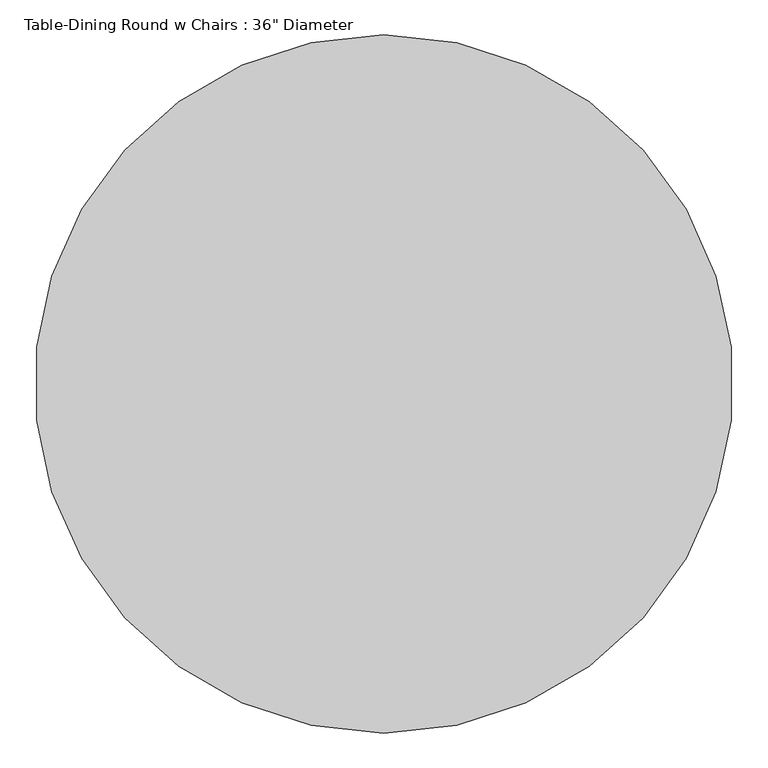
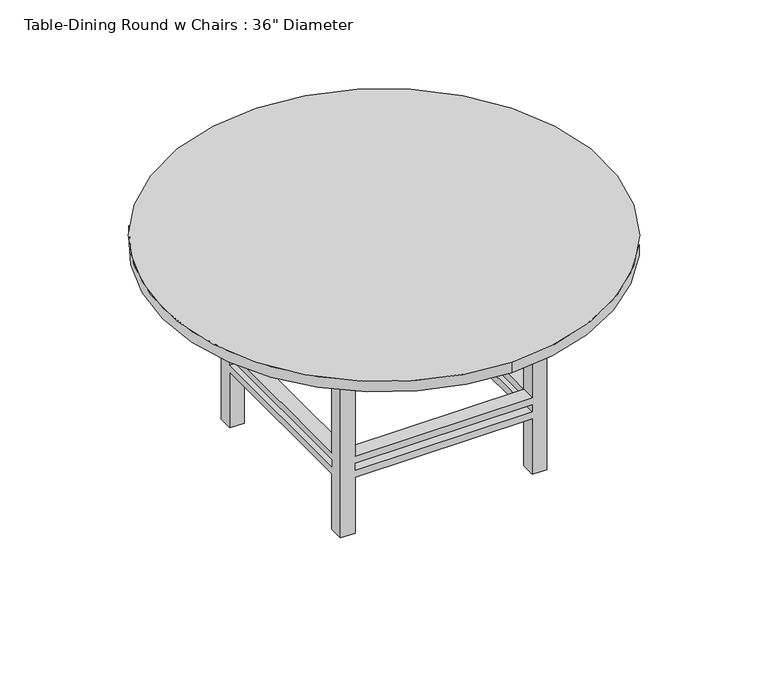
"""IFC4 building model written with IfcOpenShell, lengths in millimetres: furniture geometry."""

from ifc_helpers import new_model, si_unit, point, frame, frame_2d, origin, place, context, project, spatial, polyline, circle_curve, trimmed, segment, composite_curve, outline, extrude, faceted_brep, source, transform, mapped, element, save


def furniture_bbcc68ce(model_context):
    return source(origin(), model_context, "Body", "SolidModel", [
        faceted_brep([(408.4819672, 119.9213115, 279.4), (408.4819672, -489.6786885, 279.4), (459.2819672, -489.6786885, 279.4), (459.2819672, 119.9213115, 279.4), (-201.1180328, -489.6786885, 279.4), (-201.1180328, -540.4786885, 279.4), (408.4819672, -540.4786885, 279.4), (-201.1180328, 119.9213115, 279.4), (-251.9180328, 119.9213115, 279.4), (-251.9180328, -489.6786885, 279.4), (408.4819672, 170.7213115, 279.4), (-201.1180328, 170.7213115, 279.4), (408.4819672, 119.9213115, 254.0), (-201.1180328, 119.9213115, 254.0), (-201.1180328, 170.7213115, 254.0), (408.4819672, 170.7213115, 254.0), (-201.1180328, -489.6786885, 254.0), (-251.9180328, -489.6786885, 254.0), (-251.9180328, 119.9213115, 254.0), (408.4819672, -489.6786885, 254.0), (408.4819672, -540.4786885, 254.0), (-201.1180328, -540.4786885, 254.0), (459.2819672, 119.9213115, 254.0), (459.2819672, -489.6786885, 254.0), (-251.9180328, 170.7213115, 647.7), (-201.1180328, 170.7213115, 647.7), (408.4819672, 170.7213115, 647.7), (459.2819672, 170.7213115, 647.7), (459.2819672, 170.7213115, 0.0), (408.4819672, 170.7213115, 0.0), (408.4819672, 170.7213115, 203.2), (-201.1180328, 170.7213115, 203.2), (-201.1180328, 170.7213115, 0.0), (-251.9180328, 170.7213115, 0.0), (-201.1180328, 170.7213115, 228.6), (408.4819672, 170.7213115, 228.6), (-251.9180328, 119.9213115, 647.7), (-251.9180328, 119.9213115, 0.0), (-251.9180328, 119.9213115, 203.2), (-251.9180328, -489.6786885, 203.2), (-251.9180328, -489.6786885, 0.0), (-251.9180328, -540.4786885, 0.0), (-251.9180328, -540.4786885, 647.7), (-251.9180328, -489.6786885, 647.7), (-251.9180328, -489.6786885, 228.6), (-251.9180328, 119.9213115, 228.6), (459.2819672, -540.4786885, 647.7), (408.4819672, -540.4786885, 647.7), (-201.1180328, -540.4786885, 647.7), (-201.1180328, -540.4786885, 0.0), (-201.1180328, -540.4786885, 203.2), (408.4819672, -540.4786885, 203.2), (408.4819672, -540.4786885, 0.0), (459.2819672, -540.4786885, 0.0), (408.4819672, -540.4786885, 228.6), (-201.1180328, -540.4786885, 228.6), (459.2819672, 119.9213115, 647.7), (459.2819672, -489.6786885, 647.7), (459.2819672, -489.6786885, 0.0), (459.2819672, -489.6786885, 203.2), (459.2819672, 119.9213115, 203.2), (459.2819672, 119.9213115, 0.0), (459.2819672, 119.9213115, 228.6), (459.2819672, -489.6786885, 228.6), (-201.1180328, 119.9213115, 647.7), (408.4819672, -489.6786885, 647.7), (408.4819672, 119.9213115, 647.7), (-201.1180328, -489.6786885, 647.7), (408.4819672, 119.9213115, 0.0), (-201.1180328, -489.6786885, 0.0), (-201.1180328, 119.9213115, 0.0), (408.4819672, -489.6786885, 0.0), (-201.1180328, 119.9213115, 228.6), (-201.1180328, 119.9213115, 203.2), (408.4819672, 119.9213115, 228.6), (408.4819672, 119.9213115, 203.2), (408.4819672, -489.6786885, 228.6), (408.4819672, -489.6786885, 203.2), (-201.1180328, -489.6786885, 228.6), (-201.1180328, -489.6786885, 203.2)], [[[0, 1, 2, 3]], [[1, 4, 5, 6]], [[4, 7, 8, 9]], [[7, 0, 10, 11]], [[12, 13, 14, 15]], [[13, 16, 17, 18]], [[16, 19, 20, 21]], [[19, 12, 22, 23]], [[24, 25, 11, 10, 26, 27, 28, 29, 30, 31, 32, 33], [14, 34, 35, 15]], [[36, 24, 33, 37, 38, 39, 40, 41, 42, 43, 9, 8], [17, 44, 45, 18]], [[46, 47, 6, 5, 48, 42, 41, 49, 50, 51, 52, 53], [20, 54, 55, 21]], [[28, 27, 56, 3, 2, 57, 46, 53, 58, 59, 60, 61], [22, 62, 63, 23]], [[1, 0, 12, 19]], [[4, 1, 19, 16]], [[7, 4, 16, 13]], [[0, 7, 13, 12]], [[25, 24, 36, 64]], [[47, 46, 57, 65]], [[26, 66, 56, 27]], [[48, 67, 43, 42]], [[29, 28, 61, 68]], [[49, 41, 40, 69]], [[32, 70, 37, 33]], [[52, 71, 58, 53]], [[13, 18, 45, 72]], [[64, 36, 8, 7]], [[37, 70, 73, 38]], [[14, 13, 72, 34]], [[25, 64, 7, 11]], [[70, 32, 31, 73]], [[12, 15, 35, 74]], [[66, 26, 10, 0]], [[29, 68, 75, 30]], [[22, 12, 74, 62]], [[56, 66, 0, 3]], [[68, 61, 60, 75]], [[19, 23, 63, 76]], [[65, 57, 2, 1]], [[58, 71, 77, 59]], [[20, 19, 76, 54]], [[47, 65, 1, 6]], [[71, 52, 51, 77]], [[16, 21, 55, 78]], [[67, 48, 5, 4]], [[49, 69, 79, 50]], [[17, 16, 78, 44]], [[43, 67, 4, 9]], [[69, 40, 39, 79]], [[74, 76, 63, 62]], [[76, 78, 55, 54]], [[78, 72, 45, 44]], [[72, 74, 35, 34]], [[75, 73, 31, 30]], [[73, 79, 39, 38]], [[79, 77, 51, 50]], [[77, 75, 60, 59]], [[76, 74, 75, 77]], [[78, 76, 77, 79]], [[72, 78, 79, 73]], [[74, 72, 73, 75]]]),
        extrude(outline(polyline([(484.6819672, 196.1213115), (484.6819672, -565.8786885), (-277.3180328, -565.8786885), (-277.3180328, 196.1213115), (484.6819672, 196.1213115)]), holes=[polyline([(459.2819672, 170.7213115), (-251.9180328, 170.7213115), (-251.9180328, -540.4786885), (459.2819672, -540.4786885), (459.2819672, 170.7213115)])]), frame((0.0, 0.0, 647.7), z_axis=(0.0, 0.0, 1.0), x_axis=(1.0, 0.0, 0.0)), (0.0, 0.0, 1.0), 76.2),
        extrude(outline(composite_curve([segment(trimmed(circle_curve(frame_2d((103.6819672, -184.8786885)), 762.0), [point((103.6819672, -946.8786885))], [point((103.6819672, 577.1213115))], False, "CARTESIAN"), True, "CONTINUOUS"), segment(trimmed(circle_curve(frame_2d((103.6819672, -184.8786885)), 762.0), [point((103.6819672, 577.1213115))], [point((103.6819672, -946.8786885))], False, "CARTESIAN"), True, "CONTINUOUS")], self_intersect=False)), frame((0.0, 0.0, 723.9), z_axis=(0.0, 0.0, 1.0), x_axis=(1.0, 0.0, 0.0)), (0.0, 0.0, 1.0), 38.1),
    ])


if __name__ == "__main__":
    model = new_model("IFC4")
    model_context = context("Model", 3, world=origin())
    ifc_project = project(units=[si_unit("LENGTHUNIT", "METRE", prefix="MILLI")], contexts=[model_context])
    site = spatial("IfcSite", under=ifc_project)
    building = spatial("IfcBuilding", under=site)
    placement = place(None, origin())
    furniture_shape = furniture_bbcc68ce(model_context)
    element("IfcFurniture", 1, ObjectType="Table-Dining Round w Chairs : 36\" Diameter", at=placement, inside=building, context=model_context, shape_type="MappedRepresentation", body=[
        mapped(furniture_shape, transform((0.0, 0.0, 0.0), x_axis=(1.0, 0.0, 0.0), y_axis=(0.0, 1.0, 0.0), z_axis=(0.0, 0.0, 1.0))),
    ])
    save(model, "model.ifc")

# Revit data of these elements
# Type "Table-Dining Round w Chairs : 36\" Diameter"
#   Assembly Code = "E2020200"
#   Radius = 2' - 6"
#   Diameter = 5' - 0"
#   Height = 2' - 6"
#   Chairs = 8
#   Base Material = Pine
#   Top Material = Laminate, Linen, Matte
#   Default Elevation = 0
# Element 1 (IfcFurniture, "Table-Dining Round w Chairs : 36\" Diameter")
#   Materials on its faces: "Pine", "Laminate, Linen, Matte"
# Materials
#   "Pine": class "Wood", colour RGB 223 192 134, transparency 0, Description = "Pinus Echinata", Cost = 0
#   "Laminate, Linen, Matte": class "Plastic", colour RGB 249 239 230, transparency 0, Description = "Plastic Laminate - Linen, Matte", Cost = 0
